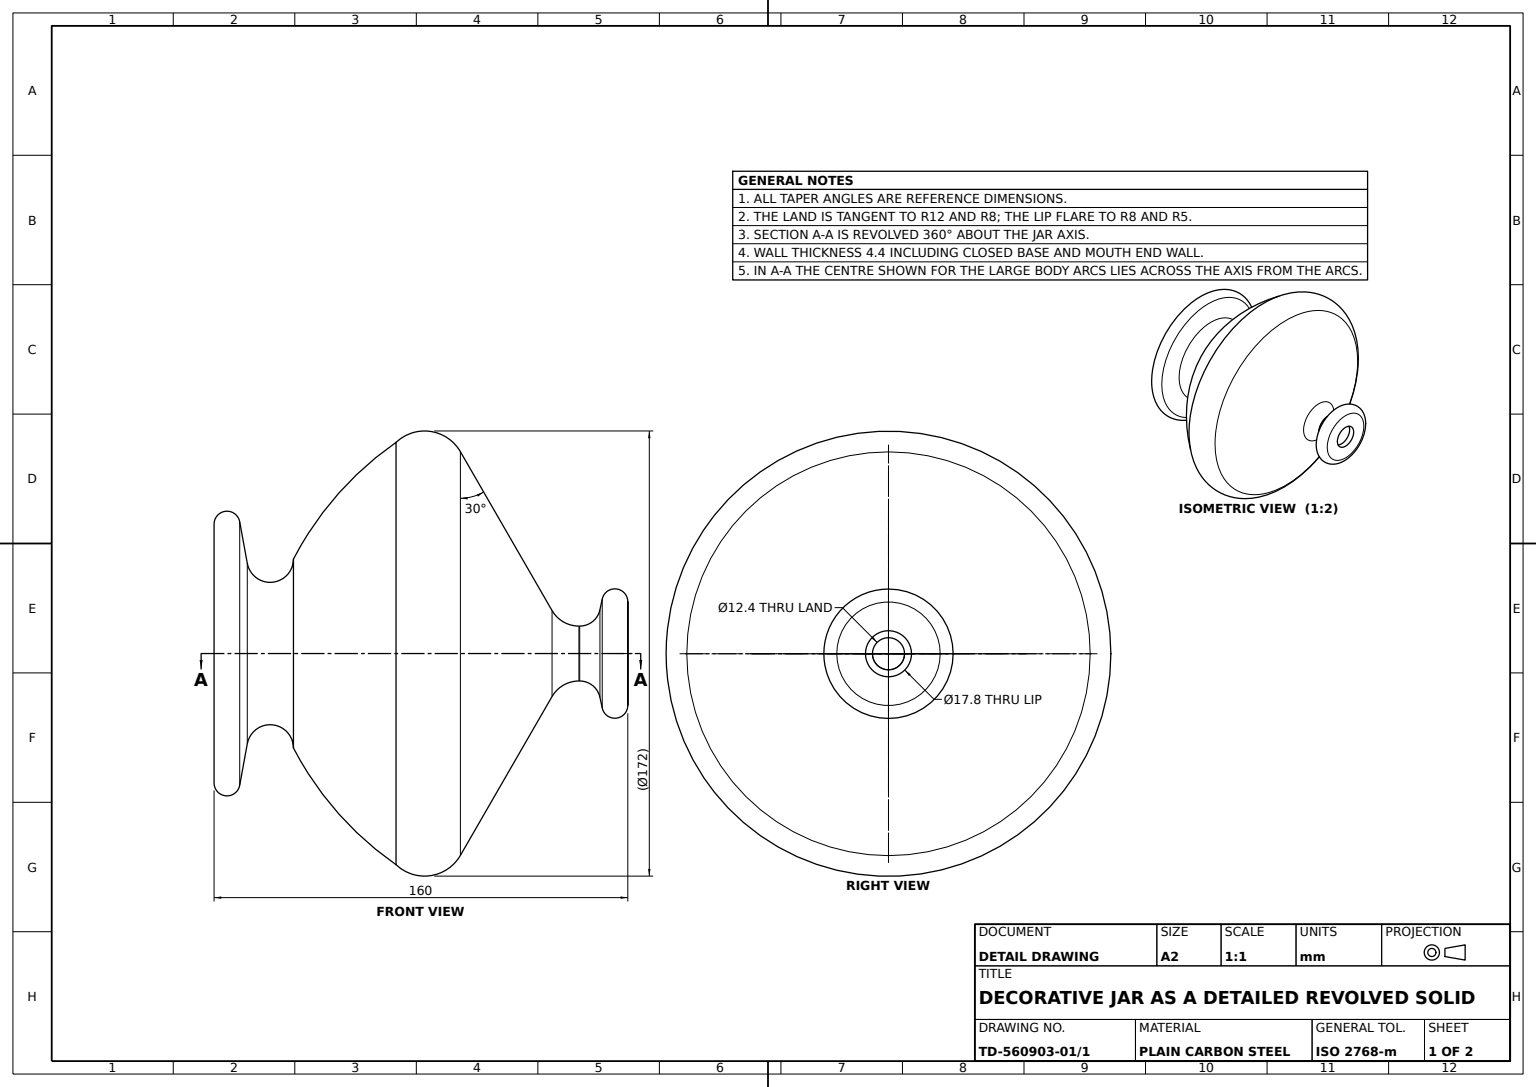
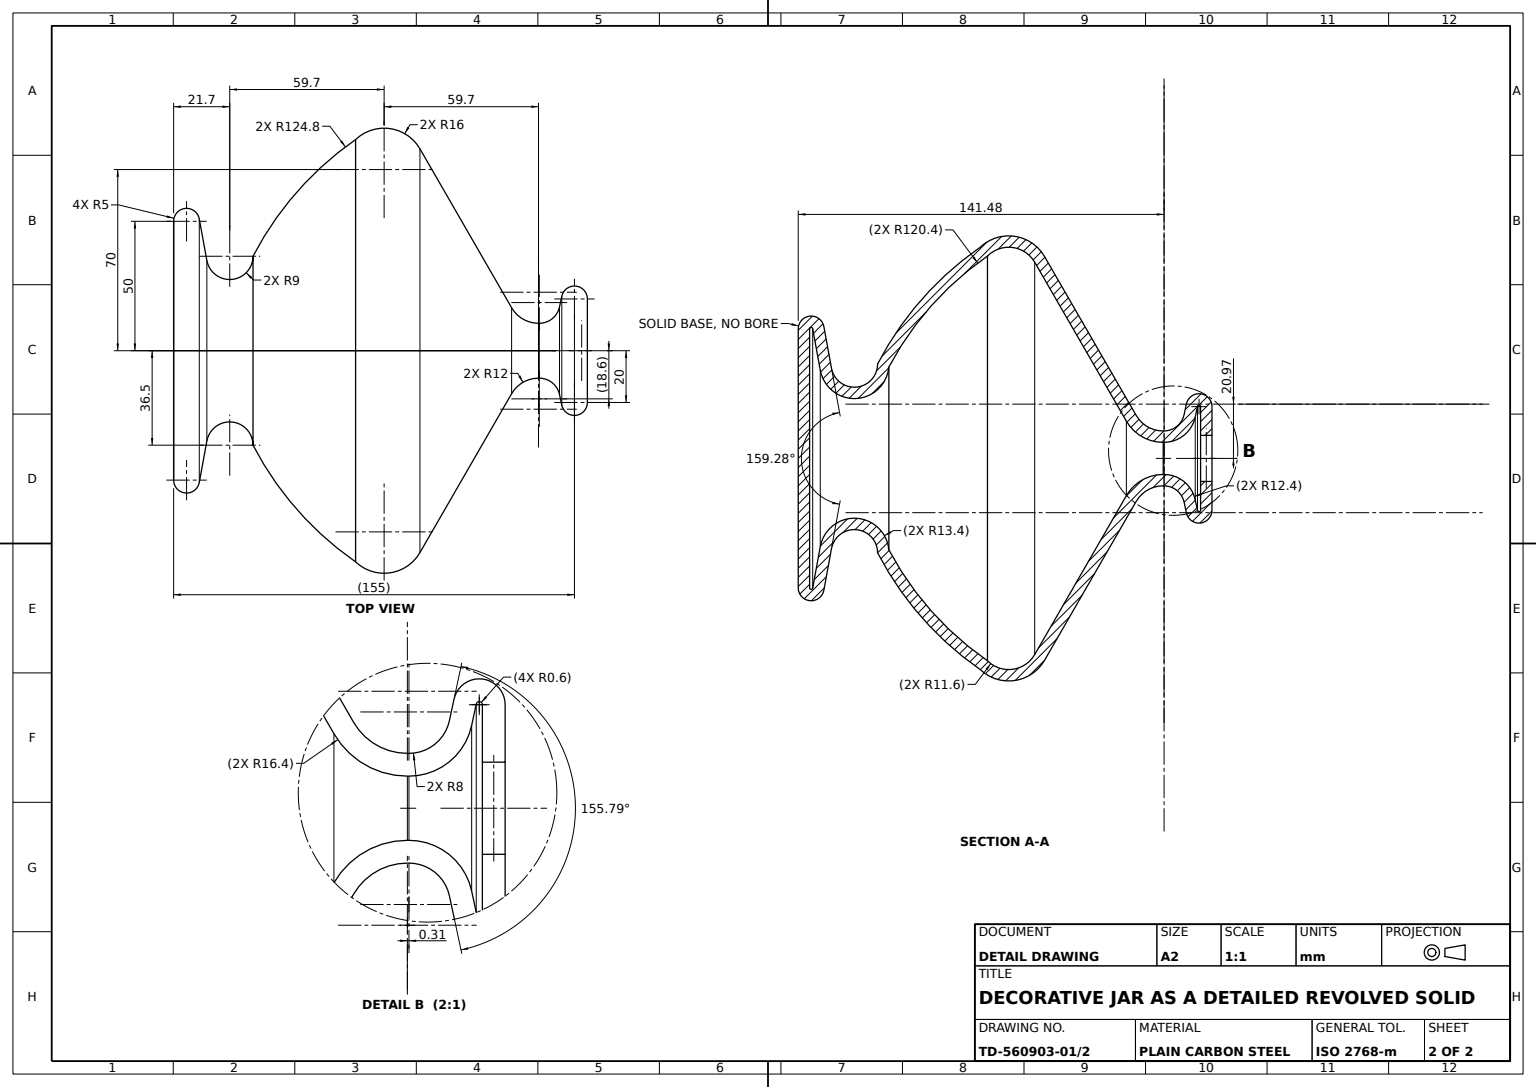
from build123d import *


with BuildPart() as part:
    # Jar Profile Sketch → Jar Body Revolve 360° (revolve)
    with BuildSketch(Plane.XY, mode=Mode.PRIVATE) as jar_body_revolve_360_sk:
        with BuildLine():
            Line((0, 0), (-50, 0))
            ThreePointArc((-50, 0), (-54.979579786, 4.548574314), (-50.899164089, 9.91848594))
            Line((-50.899164089, 9.91848594), (-34.88150464, 12.846725308))
            ThreePointArc((-34.88150464, 12.846725308), (-27.536756384, 22.512566235), (-36.5, 30.7))
            ThreePointArc((-36.5, 30.7), (-61.466698286, 47.781964835), (-81.589834313, 70.369327283))
            ThreePointArc((-81.589834313, 70.369327283), (-85.836100518, 83.684276777), (-78, 95.256406461))
            Line((-78, 95.256406461), (-16.6, 130.705712989))
            ThreePointArc((-16.6, 130.705712989), (-12.207695155, 135.098017834), (-10.6, 141.098017834))
            Line((-10.6, 141.098017834), (-10.6, 141.403935942))
            ThreePointArc((-10.6, 141.403935942), (-12.378120882, 146.43267537), (-16.92205506, 149.225988152))
            Line((-16.92205506, 149.225988152), (-21.048715588, 150.111217369))
            ThreePointArc((-21.048715588, 150.111217369), (-24.972117917, 155.527298228), (-20, 160))
            Line((-20, 160), (-8.9, 160))
            Line((-8.9, 160), (-8.9, 155.6))
            Line((-8.9, 155.6), (-20, 155.6))
            ThreePointArc((-20, 155.6), (-20.59665415, 155.063275787), (-20.125845871, 154.413346084))
            Line((-20.125845871, 154.413346084), (-15.999185343, 153.528116868))
            ThreePointArc((-15.999185343, 153.528116868), (-8.956087367, 149.198482056), (-6.2, 141.403935942))
            Line((-6.2, 141.403935942), (-6.2, 141.098017834))
            ThreePointArc((-6.2, 141.098017834), (-8.397183378, 132.898017834), (-14.4, 126.895201212))
            Line((-14.4, 126.895201212), (-75.8, 91.445894684))
            ThreePointArc((-75.8, 91.445894684), (-81.502684952, 82.899412851), (-78.181458219, 73.176634423))
            ThreePointArc((-78.181458219, 73.176634423), (-59.053725287, 51.521933043), (-35.317733129, 35.047743069))
            ThreePointArc((-35.317733129, 35.047743069), (-23.114320726, 22.319346728), (-34.090240242, 8.518457681))
            Line((-34.090240242, 8.518457681), (-50.107899691, 5.590218313))
            ThreePointArc((-50.107899691, 5.590218313), (-50.597549574, 4.945828918), (-50, 4.4))
            Line((-50, 4.4), (0, 4.4))
            Line((0, 4.4), (0, 0))
        make_face()
    revolve(jar_body_revolve_360_sk.sketch.rotate(Axis((0, 194.540686074, 0), (0, -1, 0)), 270), axis=Axis((0, 194.540686074, 0), (0, -1, 0)))


solid = part.part
